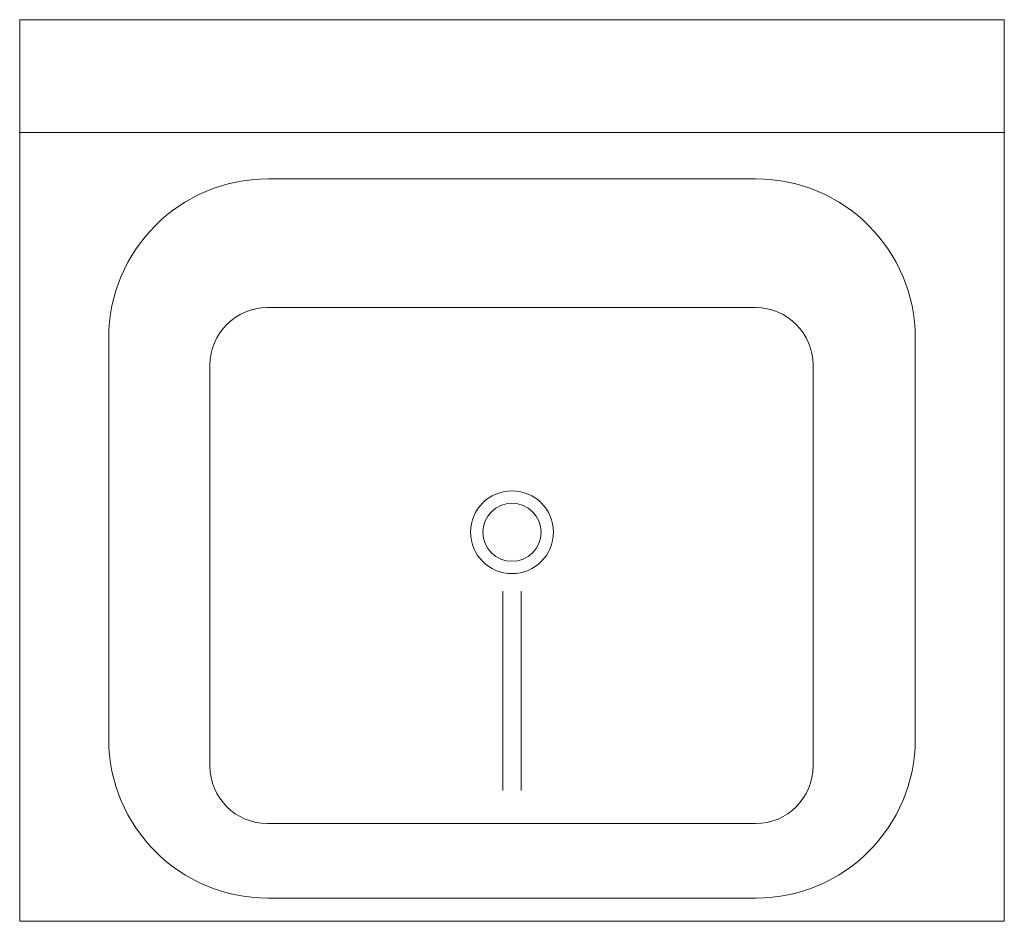
# Model space of a CAD drawing. Units: inches. Extents: x -26 to 13070, y -956 to 6917.
# Tile 13 of 13: x 12415 to 13070, y 5557 to 6157. Entities that reach past the tile are written whole.
import ezdxf

# ---------------------------------------------------------------- set-up
doc = ezdxf.new("R2010")
doc.units = ezdxf.units.IN
doc.header["$MEASUREMENT"] = 0
doc.layers.add('A-FLOR-FIXT', color=9, linetype='Continuous', lineweight=18)

# ---------------------------------------------------------------- blocks, each defined once
blk = doc.blocks.new('М14 600х655')
for p, q in [((-655, 600), (-655, 0)), ((-655, 600), (-655, 0)), ((-655, 0), (-655, 600)), ((0, 600), (-655, 600)), ((0, 0), (0, 600)), ((0, 525), (-655, 525)), ((-165.12, 494.05), (-489.88, 494.05)), ((-165.43, 408.39), (-490.19, 408.39)), ((-595.78, 388.15), (-595.78, 121.32)), ((-59.22, 121.32), (-59.22, 388.15)), ((-528.43, 370.14), (-528.43, 103.31)), ((-127.19, 103.31), (-127.19, 370.14)), ((-333.51, 87.11), (-333.51, 219.65)), ((-321.49, 87.11), (-321.49, 219.65)), ((-490.19, 65.07), (-165.43, 65.07)), ((-489.88, 15.41), (-165.12, 15.41)), ((-655, 0), (-655, 0)), ((-655, 0), (-655, 0)), ((-655, 0), (0, 0)), ((-655, 0), (0, 0))]:
    blk.add_line(p, q)
for radius in [27.55, 19.33]:
    blk.add_circle((-327.5, 258.9), radius)
for centre, radius, start, end in [((-489.88, 388.15), 105.9, 90, 180), ((-165.12, 388.15), 105.9, 0, 90), ((-490.19, 370.14), 38.24, 90, 180), ((-165.43, 370.14), 38.24, 0, 90), ((-489.88, 121.32), 105.9, 180, 270), ((-165.12, 121.32), 105.9, 270, 0), ((-490.19, 103.31), 38.24, 180, 270), ((-165.43, 103.31), 38.24, 270, 0)]:
    blk.add_arc(centre, radius, start, end)

msp = doc.modelspace()

# ---------------------------------------------------------------- block references
at = {"layer": 'A-FLOR-FIXT'}
msp.add_blockref('М14 600х655', (13070.388, 5557.21), dxfattribs=at)

doc.saveas('drawing.dxf')
